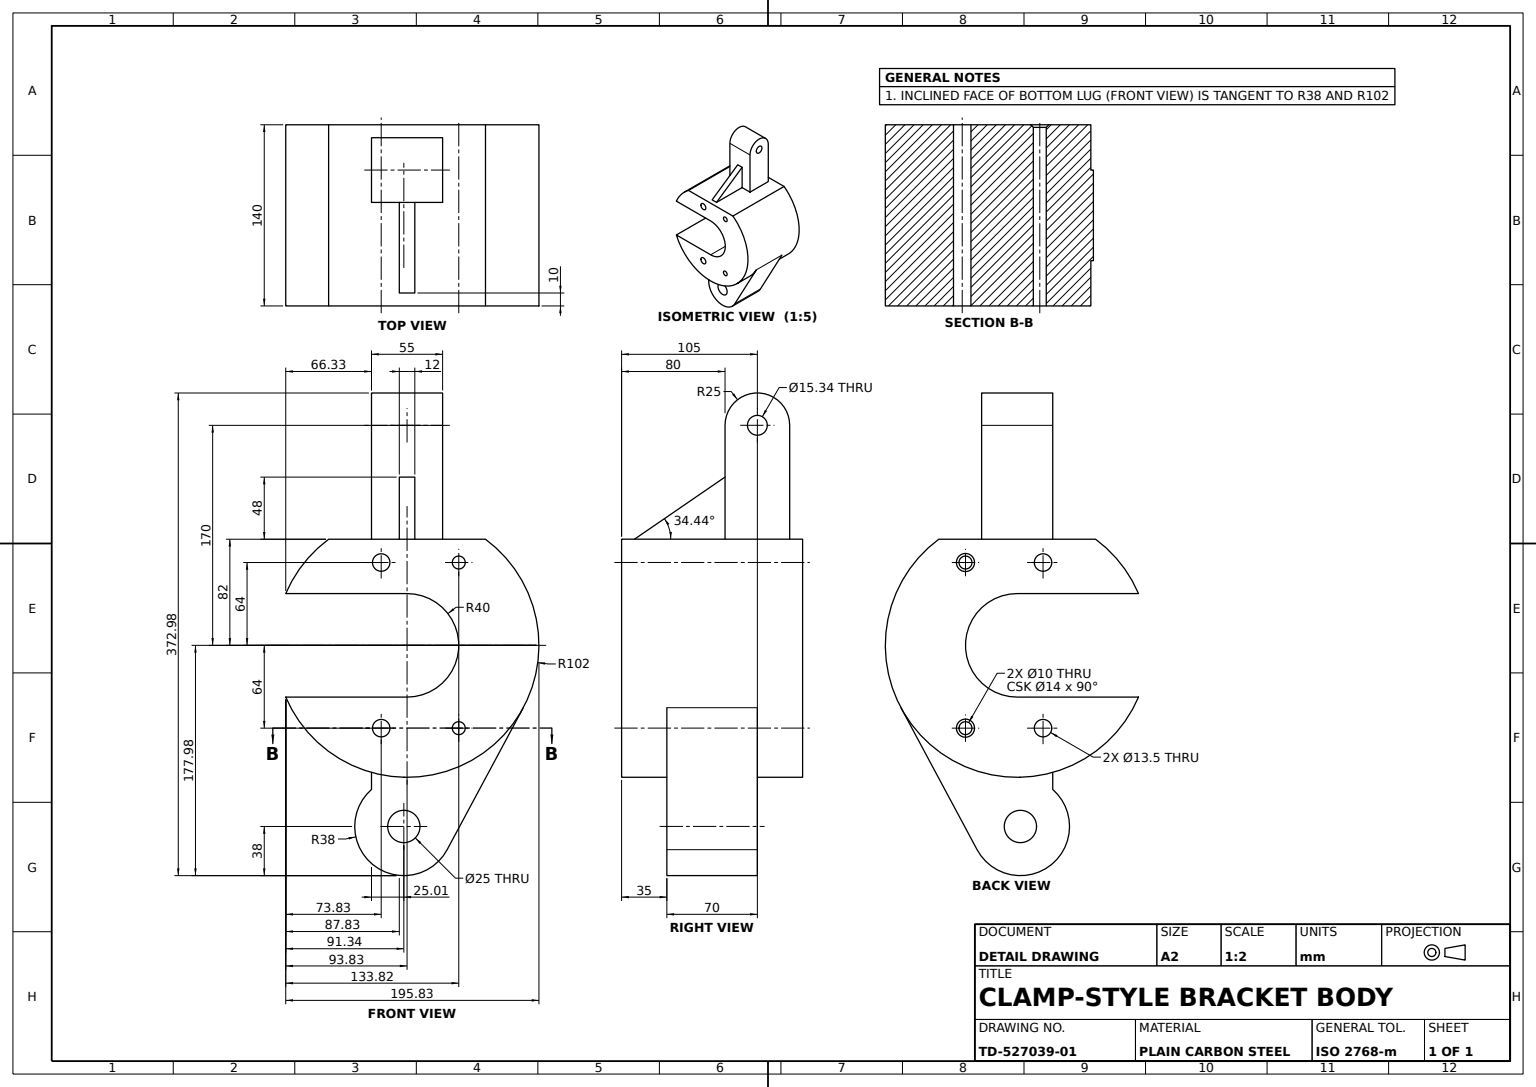
from build123d import *

# Parameters (mm, degrees)
CLAMP_BODY_PROFILE_R      = 5
CLAMP_BODY_PROFILE_R_2    = 6.75
CLAMP_BODY_DEPTH          = 70
TOP_LUG_AND_RIB_PROFILE_R = 7.668976578
TOP_LUG_DEPTH             = 27.5
GUSSET_RIB_DEPTH          = 6
BOTTOM_LUG_DEPTH          = 35
EDGE_CHAMFER_2X45_SIZE    = 2


with BuildPart() as part:
    # Clamp Body Profile → Clamp Body (new, symmetric)
    with BuildSketch(Plane.XY):
        with BuildLine():
            Line((0, -40), (-93.829632846, -40))
            ThreePointArc((-93.829632846, -40), (63.213972543, -80.04994488), (60.663003552, 82))
            Line((60.663003552, 82), (-60.663003552, 82))
            ThreePointArc((-60.663003552, 82), (-80.04994488, 63.213972543), (-93.829632846, 40))
            Line((-93.829632846, 40), (0, 40))
            ThreePointArc((0, 40), (40, 0), (0, -40))
        make_face()
        with Locations((39.991638522, 64)):
            Circle(CLAMP_BODY_PROFILE_R, mode=Mode.SUBTRACT)
        with Locations((-20, 64)):
            Circle(CLAMP_BODY_PROFILE_R_2, mode=Mode.SUBTRACT)
        with Locations(Location((39.991638522, -64, 0), (0, 0, 180))):
            Circle(CLAMP_BODY_PROFILE_R, mode=Mode.SUBTRACT)
        with Locations(Location((-20, -64, 0), (0, 0, 180))):
            Circle(CLAMP_BODY_PROFILE_R_2, mode=Mode.SUBTRACT)
    extrude(amount=CLAMP_BODY_DEPTH, both=True)

    # Top Lug and Rib Profile → Top Lug (add, symmetric)
    with BuildSketch(Plane(origin=(0, 0, 0), x_dir=(0, 0, -1), z_dir=(1, 0, 0))):
        with BuildLine():
            Line((60, 82), (60, 170))
            ThreePointArc((60, 170), (35, 195), (10, 170))
            Line((10, 170), (10, 130))
            Line((10, 130), (10, 82))
            Line((10, 82), (60, 82))
        make_face()
        with Locations((35, 170)):
            Circle(TOP_LUG_AND_RIB_PROFILE_R, mode=Mode.SUBTRACT)
    extrude(amount=TOP_LUG_DEPTH, both=True)

    # Sketch6_3 → Gusset Rib (add, symmetric)
    with BuildSketch(Plane(origin=(0, 0, 0), x_dir=(0, 0, -1), z_dir=(1, 0, 0))):
        Polygon((-60, 82), (10, 82), (10, 130), align=None)
    extrude(amount=GUSSET_RIB_DEPTH, both=True)

    # Bottom Lug Profile → Bottom Lug (add, symmetric)
    with BuildSketch(Plane.XY):
        with BuildLine():
            ThreePointArc((-27.5, -111.367680386), (-26.163106523, -169.703640044), (30.991702616, -157.947821666))
            Line((30.991702616, -157.947821666), (89.874157687, -48.235213071))
            ThreePointArc((89.874157687, -48.235213071), (51.583370989, -87.995203491), (-1.814745181, -101.983855094))
            ThreePointArc((-1.814745181, -101.983855094), (-2.152772572, -101.979344048), (-2.490826719, -101.977840326))
            Line((-2.490826719, -101.977840326), (-2.490826719, -101.969582633))
            ThreePointArc((-2.490826719, -101.969582633), (-15.1119726, -100.87431925), (-27.5, -98.222960656))
            Line((-27.5, -98.222960656), (-27.5, -111.367680386))
        make_face()
        with BuildLine():
            ThreePointArc((10.009173281, -139.977840326), (-11.329661484, -148.816675091), (-2.490826719, -127.477840326))
            ThreePointArc((-2.490826719, -127.477840326), (6.348008046, -131.139005561), (10.009173281, -139.977840326))
        make_face(mode=Mode.SUBTRACT)
    extrude(amount=BOTTOM_LUG_DEPTH, both=True)

    # Edge Chamfer 2x45
    edge_chamfer_2x45_edges = [part.edges().sort_by_distance(p)[0] for p in [
        (34.991638522, 64, -70),
        (44.991638522, -64, -70),
    ]]
    chamfer(edge_chamfer_2x45_edges, length=EDGE_CHAMFER_2X45_SIZE)


solid = part.part
